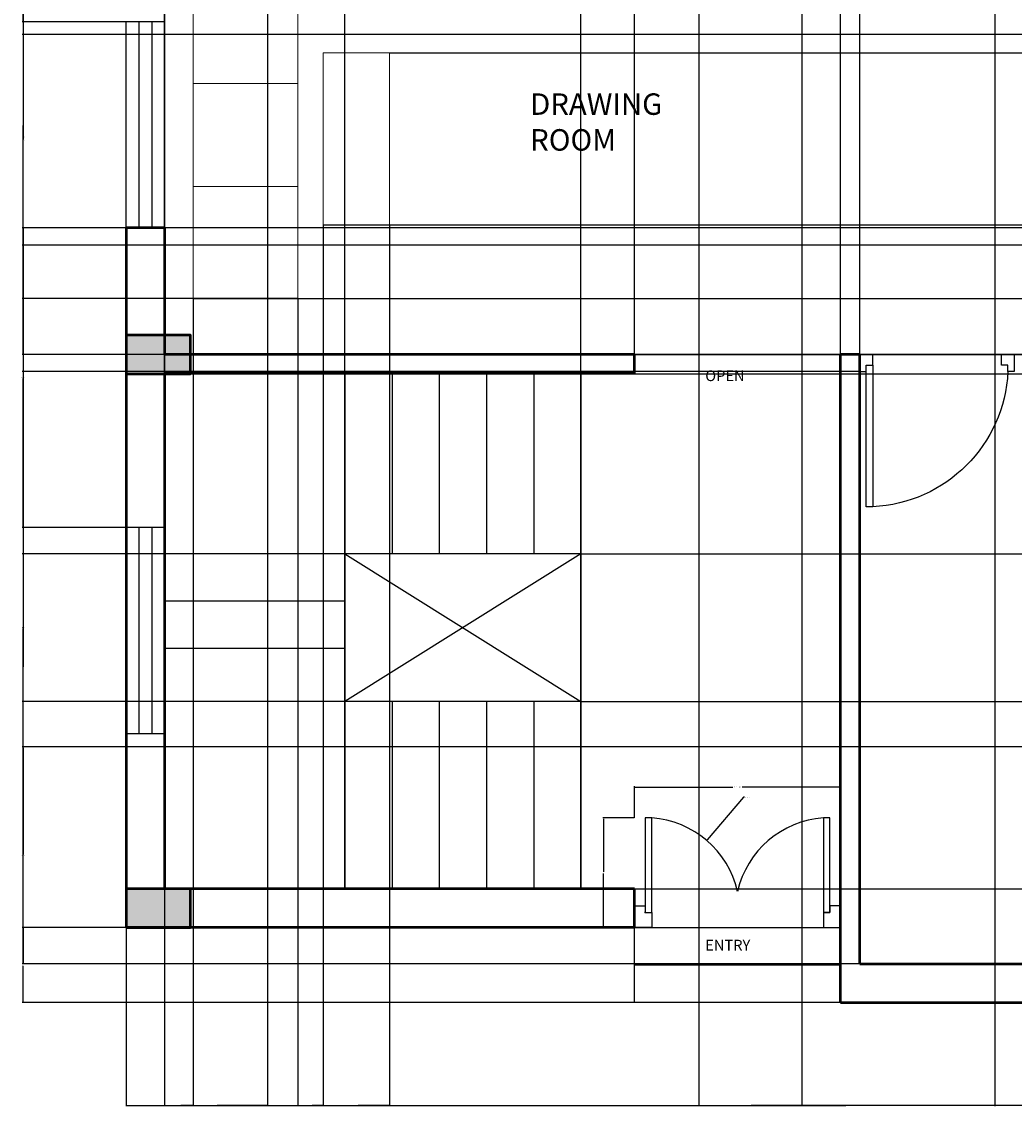
# Model space of a CAD drawing. Units: inches. Extents: x 2480 to 2840, y 795 to 1323.
# Tile 1 of 4: x 2480 to 2711, y 795 to 1047. Entities that reach past the tile are written whole.
import ezdxf

# ---------------------------------------------------------------- set-up
doc = ezdxf.new("R2010")
doc.units = ezdxf.units.IN
for name, color, linetype, lineweight in [('A-ANNO-DIMS', 2, 'Continuous', 18), ('A-ANNO-TEXT', 7, 'Continuous', 18), ('A-AREA-IDEN', 7, 'Continuous', 25), ('COLUMN', 240, 'Continuous', 50), ('door', 140, 'Continuous', 25), ('Furniture', 9, 'Continuous', 18), ('staircase', 50, 'Continuous', 25), ('wall', 7, 'Continuous', 50), ('window', 201, 'Continuous', 25)]:
    doc.layers.add(name, color=color, linetype=linetype, lineweight=lineweight)
doc.styles.get("Standard").update_dxf_attribs({"font": 'arial.ttf'})
doc.dimstyles.get("Standard").update_dxf_attribs({"dimtxt": 0.18, "dimasz": 0.18, "dimexe": 0.18, "dimexo": 0.0625, "dimgap": 0.09, "dimtad": 0, "dimtih": 1, "dimtoh": 1, "dimdec": 4, "dimzin": 0, "dimdsep": 46, "dimtxsty": 'Standard', "dimcen": 0.09, "dimadec": 0, "dimazin": 0, "dimtfac": 1, "dimtdec": 4, "dimtofl": 0, "dimtmove": 0, "dimatfit": 3, "dimfxl": 1, "dimtolj": 1, "dimtzin": 0, "dimarcsym": 0})

# ---------------------------------------------------------------- blocks, each defined once
blk = doc.blocks.new('d3')
at = {"layer": 'door'}
blk.add_line((3146.77, 1027.98), (3194.77, 1027.98), dxfattribs=at)
for points in [[(3149.27, 1031.48), (3150.77, 1031.48), (3150.77, 1053.48), (3149.27, 1053.48)], [(3190.77, 1031.48), (3192.27, 1031.48), (3192.27, 1053.48), (3190.77, 1053.48)]]:
    blk.add_lwpolyline(points, close=True, dxfattribs=at)
for points in [[(3150.77, 1027.98), (3146.77, 1027.98), (3146.77, 1032.98), (3149.27, 1032.98), (3149.27, 1031.48), (3150.77, 1031.48), (3150.77, 1027.98)], [(3190.77, 1027.98), (3194.77, 1027.98), (3194.77, 1032.98), (3192.27, 1032.98), (3192.27, 1031.48), (3190.77, 1031.48), (3190.77, 1027.98)]]:
    blk.add_lwpolyline(points, dxfattribs=at)
for centre, start, end in [((3149.27, 1031.48), 12.8362, 86.0995), ((3192.27, 1031.48), 93.9005, 167.1638)]:
    blk.add_arc(centre, 22.05, start, end, dxfattribs=at)
blk = doc.blocks.new('w1')
at = {"layer": 'window'}
for p, q in [((2922.2, 1100.57), (2922.2, 1052.57)), ((2925.2, 1100.57), (2925.2, 1052.57))]:
    blk.add_line(p, q, dxfattribs=at)
blk.add_lwpolyline([(2919.2, 1052.57), (2928.2, 1052.57), (2928.2, 1100.57), (2919.2, 1100.57)], close=True, dxfattribs=at)
blk = doc.blocks.new('d1')
at = {"layer": 'door'}
blk.add_line((3049.73, 1052.02), (3085.73, 1052.02), dxfattribs=at)
blk.add_lwpolyline([(3051.23, 1054.52), (3052.73, 1054.52), (3052.73, 1087.52), (3051.23, 1087.52)], close=True, dxfattribs=at)
for points in [[(3052.73, 1052.02), (3049.73, 1052.02), (3049.73, 1056.02), (3051.23, 1056.02), (3051.23, 1054.52), (3052.73, 1054.52), (3052.73, 1052.02)], [(3082.73, 1052.02), (3085.73, 1052.02), (3085.73, 1056.02), (3084.23, 1056.02), (3084.23, 1054.52), (3082.73, 1054.52), (3082.73, 1052.02)]]:
    blk.add_lwpolyline(points, dxfattribs=at)
blk.add_arc((3051.23, 1054.52), 33.03, 2.6026, 87.3974, dxfattribs=at)
blk = doc.blocks.new('C')
at = {"layer": 'COLUMN'}
h = blk.add_hatch(color=256, dxfattribs=at)
h.dxf.hatch_style = 1
h.paths.add_polyline_path([(3016.24, 1218.72), (3031.24, 1218.72), (3031.24, 1227.72), (3016.24, 1227.72)])
blk.add_lwpolyline([(3016.24, 1218.72), (3031.24, 1218.72), (3031.24, 1227.72), (3016.24, 1227.72)], close=True, dxfattribs=at)
blk = doc.blocks.new('*D22')
at = {"layer": 'A-ANNO-DIMS', "color": 0, "lineweight": -2, "transparency": 16777216}
for p, q in [((2622.45, 861.8), (2622.45, 869.12)), ((2622.63, 868.94), (2645.37, 868.94)), ((2670.27, 868.94), (2647.54, 868.94)), ((2670.45, 861.8), (2670.45, 869.12))]:
    blk.add_line(p, q, dxfattribs=at)
at = {"layer": 'A-ANNO-DIMS', "color": 0, "transparency": 16777216}
for points in [[(2622.63, 868.97), (2622.63, 868.91), (2622.45, 868.94)], [(2670.27, 868.97), (2670.27, 868.91), (2670.45, 868.94)]]:
    blk.add_solid(points, dxfattribs=at)
at = {"layer": 'Defpoints', "color": 0, "transparency": 16777216}
for p in [(2670.45, 868.94), (2622.45, 861.74), (2670.45, 861.74)]:
    blk.add_point(p, dxfattribs=at)
at = {"layer": 'A-ANNO-DIMS', "color": 0, "transparency": 16777216, "insert": (2646.45, 868.94), "char_height": 0.18, "attachment_point": 5}
blk.add_mtext('\\A1;ENTRY DOOR 48', dxfattribs=at)
blk = doc.blocks.new('*D23')
at = {"layer": 'A-ANNO-DIMS', "color": 0, "lineweight": -2, "transparency": 16777216}
for p, q in [((2622.39, 861.74), (2615.07, 861.74)), ((2615.25, 861.56), (2615.25, 849.17)), ((2615.25, 836.42), (2615.25, 848.81)), ((2622.39, 836.24), (2615.07, 836.24))]:
    blk.add_line(p, q, dxfattribs=at)
at = {"layer": 'A-ANNO-DIMS', "color": 0, "transparency": 16777216}
for points in [[(2615.22, 861.56), (2615.28, 861.56), (2615.25, 861.74)], [(2615.22, 836.42), (2615.28, 836.42), (2615.25, 836.24)]]:
    blk.add_solid(points, dxfattribs=at)
at = {"layer": 'Defpoints', "color": 0, "transparency": 16777216}
for p in [(2615.25, 861.74), (2622.45, 861.74), (2622.45, 836.24)]:
    blk.add_point(p, dxfattribs=at)
at = {"layer": 'A-ANNO-DIMS', "color": 0, "transparency": 16777216, "insert": (2615.25, 848.99), "char_height": 0.18, "attachment_point": 5}
blk.add_mtext('\\A1;26', dxfattribs=at)
blk = doc.blocks.new('*D28')
at = {"layer": 'A-ANNO-DIMS', "color": 0, "lineweight": -2, "transparency": 16777216}
for p, q in [((2503.95, 836.18), (2503.95, 794.56)), ((2815.95, 818.68), (2815.95, 794.56)), ((2504.13, 794.74), (2659.67, 794.74)), ((2815.77, 794.74), (2660.24, 794.74))]:
    blk.add_line(p, q, dxfattribs=at)
at = {"layer": 'A-ANNO-DIMS', "color": 0, "transparency": 16777216}
for points in [[(2504.13, 794.77), (2504.13, 794.71), (2503.95, 794.74)], [(2815.77, 794.77), (2815.77, 794.71), (2815.95, 794.74)]]:
    blk.add_solid(points, dxfattribs=at)
at = {"layer": 'Defpoints', "color": 0, "transparency": 16777216}
for p in [(2503.95, 836.24), (2815.95, 818.74), (2815.95, 794.74)]:
    blk.add_point(p, dxfattribs=at)
at = {"layer": 'A-ANNO-DIMS', "color": 0, "transparency": 16777216, "insert": (2659.95, 794.74), "char_height": 0.18, "attachment_point": 5}
blk.add_mtext('\\A1;312', dxfattribs=at)
blk = doc.blocks.new('*D35')
at = {"layer": 'A-ANNO-DIMS', "color": 0, "lineweight": -2, "transparency": 16777216}
for p, q in [((2503.89, 1105.24), (2479.77, 1105.24)), ((2479.95, 1105.06), (2479.95, 1076.42)), ((2479.95, 1047.42), (2479.95, 1076.06)), ((2503.89, 1047.24), (2479.77, 1047.24))]:
    blk.add_line(p, q, dxfattribs=at)
at = {"layer": 'A-ANNO-DIMS', "color": 0, "transparency": 16777216}
for points in [[(2479.92, 1105.06), (2479.98, 1105.06), (2479.95, 1105.24)], [(2479.92, 1047.42), (2479.98, 1047.42), (2479.95, 1047.24)]]:
    blk.add_solid(points, dxfattribs=at)
at = {"layer": 'Defpoints', "color": 0, "transparency": 16777216}
for p in [(2503.95, 1105.24), (2479.95, 1047.24), (2503.95, 1047.24)]:
    blk.add_point(p, dxfattribs=at)
at = {"layer": 'A-ANNO-DIMS', "color": 0, "transparency": 16777216, "insert": (2479.95, 1076.24), "char_height": 0.18, "attachment_point": 5}
blk.add_mtext('\\A1;58', dxfattribs=at)
blk = doc.blocks.new('*D36')
at = {"layer": 'A-ANNO-DIMS', "color": 0, "lineweight": -2, "transparency": 16777216}
for p, q in [((2503.89, 999.24), (2479.77, 999.24)), ((2479.95, 999.06), (2479.95, 964.51)), ((2479.95, 929.6), (2479.95, 964.15)), ((2503.89, 929.42), (2479.77, 929.42))]:
    blk.add_line(p, q, dxfattribs=at)
at = {"layer": 'A-ANNO-DIMS', "color": 0, "transparency": 16777216}
for points in [[(2479.92, 999.06), (2479.98, 999.06), (2479.95, 999.24)], [(2479.92, 929.6), (2479.98, 929.6), (2479.95, 929.42)]]:
    blk.add_solid(points, dxfattribs=at)
at = {"layer": 'Defpoints', "color": 0, "transparency": 16777216}
for p in [(2503.95, 999.24), (2479.95, 929.42), (2503.95, 929.42)]:
    blk.add_point(p, dxfattribs=at)
at = {"layer": 'A-ANNO-DIMS', "color": 0, "transparency": 16777216, "insert": (2479.95, 964.33), "char_height": 0.18, "attachment_point": 5}
blk.add_mtext('\\A1;69.82', dxfattribs=at)
blk = doc.blocks.new('*D37')
at = {"layer": 'A-ANNO-DIMS', "color": 0, "lineweight": -2, "transparency": 16777216}
for p, q in [((2806.89, 878.28), (2479.77, 878.28)), ((2479.95, 878.1), (2479.95, 853.19)), ((2479.95, 827.92), (2479.95, 852.83)), ((2806.89, 827.74), (2479.77, 827.74))]:
    blk.add_line(p, q, dxfattribs=at)
at = {"layer": 'A-ANNO-DIMS', "color": 0, "transparency": 16777216}
for points in [[(2479.92, 878.1), (2479.98, 878.1), (2479.95, 878.28)], [(2479.92, 827.92), (2479.98, 827.92), (2479.95, 827.74)]]:
    blk.add_solid(points, dxfattribs=at)
at = {"layer": 'Defpoints', "color": 0, "transparency": 16777216}
for p in [(2479.95, 878.28), (2806.95, 878.28), (2806.95, 827.74)]:
    blk.add_point(p, dxfattribs=at)
at = {"layer": 'A-ANNO-DIMS', "color": 0, "transparency": 16777216, "insert": (2479.95, 853.01), "char_height": 0.18, "attachment_point": 5}
blk.add_mtext('\\A1;50.53', dxfattribs=at)
blk = doc.blocks.new('*D38')
at = {"layer": 'A-ANNO-DIMS', "color": 0, "lineweight": -2, "transparency": 16777216}
for p, q in [((2806.89, 999.24), (2479.77, 999.24)), ((2479.95, 999.06), (2479.95, 984.67)), ((2479.95, 969.92), (2479.95, 984.31)), ((2806.89, 969.74), (2479.77, 969.74))]:
    blk.add_line(p, q, dxfattribs=at)
at = {"layer": 'A-ANNO-DIMS', "color": 0, "transparency": 16777216}
for points in [[(2479.92, 999.06), (2479.98, 999.06), (2479.95, 999.24)], [(2479.92, 969.92), (2479.98, 969.92), (2479.95, 969.74)]]:
    blk.add_solid(points, dxfattribs=at)
at = {"layer": 'Defpoints', "color": 0, "transparency": 16777216}
for p in [(2479.95, 999.24), (2806.95, 999.24), (2806.95, 969.74)]:
    blk.add_point(p, dxfattribs=at)
at = {"layer": 'A-ANNO-DIMS', "color": 0, "transparency": 16777216, "insert": (2479.95, 984.49), "char_height": 0.18, "attachment_point": 5}
blk.add_mtext('\\A1;29.5', dxfattribs=at)
blk = doc.blocks.new('*D42')
at = {"layer": 'A-ANNO-DIMS', "color": 0, "lineweight": -2, "transparency": 16777216}
for p, q in [((2512.95, 969.8), (2512.95, 1322.93)), ((2513.13, 1322.75), (2567.32, 1322.75)), ((2622.27, 1322.75), (2568.09, 1322.75)), ((2622.45, 969.8), (2622.45, 1322.93))]:
    blk.add_line(p, q, dxfattribs=at)
at = {"layer": 'A-ANNO-DIMS', "color": 0, "transparency": 16777216}
for points in [[(2513.13, 1322.78), (2513.13, 1322.72), (2512.95, 1322.75)], [(2622.27, 1322.78), (2622.27, 1322.72), (2622.45, 1322.75)]]:
    blk.add_solid(points, dxfattribs=at)
at = {"layer": 'Defpoints', "color": 0, "transparency": 16777216}
for p in [(2622.45, 1322.75), (2512.95, 969.74), (2622.45, 969.74)]:
    blk.add_point(p, dxfattribs=at)
at = {"layer": 'A-ANNO-DIMS', "color": 0, "transparency": 16777216, "insert": (2567.7, 1322.75), "char_height": 0.18, "attachment_point": 5}
blk.add_mtext('\\A1;109.5', dxfattribs=at)
blk = doc.blocks.new('*D43')
at = {"layer": 'A-ANNO-DIMS', "color": 0, "lineweight": -2, "transparency": 16777216}
for p, q in [((2622.39, 836.24), (2479.77, 836.24)), ((2479.95, 836.06), (2479.95, 827.67)), ((2479.95, 818.92), (2479.95, 827.31)), ((2622.39, 818.74), (2479.77, 818.74))]:
    blk.add_line(p, q, dxfattribs=at)
at = {"layer": 'A-ANNO-DIMS', "color": 0, "transparency": 16777216}
for points in [[(2479.92, 836.06), (2479.98, 836.06), (2479.95, 836.24)], [(2479.92, 818.92), (2479.98, 818.92), (2479.95, 818.74)]]:
    blk.add_solid(points, dxfattribs=at)
at = {"layer": 'Defpoints', "color": 0, "transparency": 16777216}
for p in [(2479.95, 836.24), (2622.45, 836.24), (2622.45, 818.74)]:
    blk.add_point(p, dxfattribs=at)
at = {"layer": 'A-ANNO-DIMS', "color": 0, "transparency": 16777216, "insert": (2479.95, 827.49), "char_height": 0.18, "attachment_point": 5}
blk.add_mtext('\\A1;17.5', dxfattribs=at)
blk = doc.blocks.new('*D44')
at = {"layer": 'A-ANNO-DIMS', "color": 0, "lineweight": -2, "transparency": 16777216}
for p, q in [((2706.39, 1076.74), (2479.77, 1076.74)), ((2479.95, 1076.56), (2479.95, 1023.42)), ((2479.95, 969.92), (2479.95, 1023.06)), ((2710.89, 969.74), (2479.77, 969.74))]:
    blk.add_line(p, q, dxfattribs=at)
at = {"layer": 'A-ANNO-DIMS', "color": 0, "transparency": 16777216}
for points in [[(2479.92, 1076.56), (2479.98, 1076.56), (2479.95, 1076.74)], [(2479.92, 969.92), (2479.98, 969.92), (2479.95, 969.74)]]:
    blk.add_solid(points, dxfattribs=at)
at = {"layer": 'Defpoints', "color": 0, "transparency": 16777216}
for p in [(2479.95, 1076.74), (2706.45, 1076.74), (2710.95, 969.74)]:
    blk.add_point(p, dxfattribs=at)
at = {"layer": 'A-ANNO-DIMS', "color": 0, "transparency": 16777216, "insert": (2479.95, 1023.24), "char_height": 0.18, "attachment_point": 5}
blk.add_mtext('\\A1;107', dxfattribs=at)
blk = doc.blocks.new('*D45')
at = {"layer": 'A-ANNO-DIMS', "color": 0, "lineweight": -2, "transparency": 16777216}
for p, q in [((2512.95, 923.3), (2512.95, 1322.93)), ((2513.13, 1322.75), (2533.73, 1322.75)), ((2554.77, 1322.75), (2534.18, 1322.75)), ((2554.95, 923.3), (2554.95, 1322.93))]:
    blk.add_line(p, q, dxfattribs=at)
at = {"layer": 'A-ANNO-DIMS', "color": 0, "transparency": 16777216}
for points in [[(2513.13, 1322.78), (2513.13, 1322.72), (2512.95, 1322.75)], [(2554.77, 1322.78), (2554.77, 1322.72), (2554.95, 1322.75)]]:
    blk.add_solid(points, dxfattribs=at)
at = {"layer": 'Defpoints', "color": 0, "transparency": 16777216}
for p in [(2554.95, 1322.75), (2512.95, 923.24), (2554.95, 923.24)]:
    blk.add_point(p, dxfattribs=at)
at = {"layer": 'A-ANNO-DIMS', "color": 0, "transparency": 16777216, "insert": (2533.95, 1322.75), "char_height": 0.18, "attachment_point": 5}
blk.add_mtext('\\A1;42', dxfattribs=at)
blk = doc.blocks.new('*D46')
at = {"layer": 'A-ANNO-DIMS', "color": 0, "lineweight": -2, "transparency": 16777216}
for p, q in [((2610.02, 888.87), (2840.14, 888.87)), ((2839.96, 888.69), (2839.96, 867.24)), ((2839.96, 845.42), (2839.96, 866.87)), ((2610.02, 845.24), (2840.14, 845.24))]:
    blk.add_line(p, q, dxfattribs=at)
at = {"layer": 'A-ANNO-DIMS', "color": 0, "transparency": 16777216}
for points in [[(2839.93, 888.69), (2839.99, 888.69), (2839.96, 888.87)], [(2839.93, 845.42), (2839.99, 845.42), (2839.96, 845.24)]]:
    blk.add_solid(points, dxfattribs=at)
at = {"layer": 'Defpoints', "color": 0, "transparency": 16777216}
for p in [(2609.95, 888.87), (2839.96, 888.87), (2609.95, 845.24)]:
    blk.add_point(p, dxfattribs=at)
at = {"layer": 'A-ANNO-DIMS', "color": 0, "transparency": 16777216, "insert": (2839.96, 867.06), "char_height": 0.18, "attachment_point": 5}
blk.add_mtext('\\A1;43.63', dxfattribs=at)
blk = doc.blocks.new('*D47')
at = {"layer": 'A-ANNO-DIMS', "color": 0, "lineweight": -2, "transparency": 16777216}
for p, q in [((2554.95, 845.3), (2554.95, 1322.93)), ((2555.13, 1322.75), (2582.23, 1322.75)), ((2609.77, 1322.75), (2582.67, 1322.75)), ((2609.95, 845.3), (2609.95, 1322.93))]:
    blk.add_line(p, q, dxfattribs=at)
at = {"layer": 'A-ANNO-DIMS', "color": 0, "transparency": 16777216}
for points in [[(2555.13, 1322.78), (2555.13, 1322.72), (2554.95, 1322.75)], [(2609.77, 1322.78), (2609.77, 1322.72), (2609.95, 1322.75)]]:
    blk.add_solid(points, dxfattribs=at)
at = {"layer": 'Defpoints', "color": 0, "transparency": 16777216}
for p in [(2609.95, 1322.75), (2554.95, 845.24), (2609.95, 845.24)]:
    blk.add_point(p, dxfattribs=at)
at = {"layer": 'A-ANNO-DIMS', "color": 0, "transparency": 16777216, "insert": (2582.45, 1322.75), "char_height": 0.18, "attachment_point": 5}
blk.add_mtext('\\A1;55', dxfattribs=at)
blk = doc.blocks.new('*D48')
at = {"layer": 'A-ANNO-DIMS', "color": 0, "lineweight": -2, "transparency": 16777216}
for p, q in [((2554.89, 923.24), (2479.77, 923.24)), ((2479.95, 923.06), (2479.95, 906.24)), ((2479.95, 889.05), (2479.95, 905.87)), ((2554.89, 888.87), (2479.77, 888.87))]:
    blk.add_line(p, q, dxfattribs=at)
at = {"layer": 'A-ANNO-DIMS', "color": 0, "transparency": 16777216}
for points in [[(2479.92, 923.06), (2479.98, 923.06), (2479.95, 923.24)], [(2479.92, 889.05), (2479.98, 889.05), (2479.95, 888.87)]]:
    blk.add_solid(points, dxfattribs=at)
at = {"layer": 'Defpoints', "color": 0, "transparency": 16777216}
for p in [(2479.95, 923.24), (2554.95, 923.24), (2554.95, 888.87)]:
    blk.add_point(p, dxfattribs=at)
at = {"layer": 'A-ANNO-DIMS', "color": 0, "transparency": 16777216, "insert": (2479.95, 906.06), "char_height": 0.18, "attachment_point": 5}
blk.add_mtext('\\A1;34.37', dxfattribs=at)
blk = doc.blocks.new('*D49')
at = {"layer": 'A-ANNO-DIMS', "color": 0, "lineweight": -2, "transparency": 16777216}
for p, q in [((2610.02, 965.24), (2840.14, 965.24)), ((2839.96, 965.06), (2839.96, 944.42)), ((2839.96, 923.42), (2839.96, 944.06)), ((2610.02, 923.24), (2840.14, 923.24))]:
    blk.add_line(p, q, dxfattribs=at)
at = {"layer": 'A-ANNO-DIMS', "color": 0, "transparency": 16777216}
for points in [[(2839.93, 965.06), (2839.99, 965.06), (2839.96, 965.24)], [(2839.93, 923.42), (2839.99, 923.42), (2839.96, 923.24)]]:
    blk.add_solid(points, dxfattribs=at)
at = {"layer": 'Defpoints', "color": 0, "transparency": 16777216}
for p in [(2609.95, 965.24), (2839.96, 965.24), (2609.95, 923.24)]:
    blk.add_point(p, dxfattribs=at)
at = {"layer": 'A-ANNO-DIMS', "color": 0, "transparency": 16777216, "insert": (2839.96, 944.24), "char_height": 0.18, "attachment_point": 5}
blk.add_mtext('\\A1;42', dxfattribs=at)
blk = doc.blocks.new('*D50')
at = {"layer": 'A-ANNO-DIMS', "color": 0, "lineweight": -2, "transparency": 16777216}
for p, q in [((2637.45, 1076.68), (2637.45, 794.56)), ((2706.45, 1076.68), (2706.45, 794.56)), ((2637.63, 794.74), (2671.73, 794.74)), ((2706.27, 794.74), (2672.17, 794.74))]:
    blk.add_line(p, q, dxfattribs=at)
at = {"layer": 'A-ANNO-DIMS', "color": 0, "transparency": 16777216}
for points in [[(2637.63, 794.77), (2637.63, 794.71), (2637.45, 794.74)], [(2706.27, 794.77), (2706.27, 794.71), (2706.45, 794.74)]]:
    blk.add_solid(points, dxfattribs=at)
at = {"layer": 'Defpoints', "color": 0, "transparency": 16777216}
for p in [(2637.45, 1076.74), (2706.45, 1076.74), (2706.45, 794.74)]:
    blk.add_point(p, dxfattribs=at)
at = {"layer": 'A-ANNO-DIMS', "color": 0, "transparency": 16777216, "insert": (2671.95, 794.74), "char_height": 0.18, "attachment_point": 5}
blk.add_mtext('\\A1;69', dxfattribs=at)
blk = doc.blocks.new('*D52')
at = {"layer": 'A-ANNO-DIMS', "color": 0, "lineweight": -2, "transparency": 16777216}
for p, q in [((2670.45, 818.8), (2670.45, 1322.93)), ((2670.63, 1322.75), (2672.45, 1322.75)), ((2674.77, 1322.75), (2672.96, 1322.75)), ((2674.95, 827.8), (2674.95, 1322.93))]:
    blk.add_line(p, q, dxfattribs=at)
at = {"layer": 'A-ANNO-DIMS', "color": 0, "transparency": 16777216}
for points in [[(2670.63, 1322.78), (2670.63, 1322.72), (2670.45, 1322.75)], [(2674.77, 1322.78), (2674.77, 1322.72), (2674.95, 1322.75)]]:
    blk.add_solid(points, dxfattribs=at)
at = {"layer": 'Defpoints', "color": 0, "transparency": 16777216}
for p in [(2674.95, 1322.75), (2674.95, 827.74), (2670.45, 818.74)]:
    blk.add_point(p, dxfattribs=at)
at = {"layer": 'A-ANNO-DIMS', "color": 0, "transparency": 16777216, "insert": (2672.7, 1322.75), "char_height": 0.18, "attachment_point": 5}
blk.add_mtext('\\A1;4.5', dxfattribs=at)
blk = doc.blocks.new('*D53')
at = {"layer": 'A-ANNO-DIMS', "color": 0, "lineweight": -2, "transparency": 16777216}
for p, q in [((2565.4, 1040.02), (2840.14, 1040.02)), ((2839.96, 1039.84), (2839.96, 1020.15)), ((2839.96, 1000.1), (2839.96, 1019.79)), ((2565.4, 999.92), (2840.14, 999.92))]:
    blk.add_line(p, q, dxfattribs=at)
at = {"layer": 'A-ANNO-DIMS', "color": 0, "transparency": 16777216}
for points in [[(2839.93, 1039.84), (2839.99, 1039.84), (2839.96, 1040.02)], [(2839.93, 1000.1), (2839.99, 1000.1), (2839.96, 999.92)]]:
    blk.add_solid(points, dxfattribs=at)
at = {"layer": 'Defpoints', "color": 0, "transparency": 16777216}
for p in [(2565.34, 1040.02), (2839.96, 1040.02), (2565.34, 999.92)]:
    blk.add_point(p, dxfattribs=at)
at = {"layer": 'A-ANNO-DIMS', "color": 0, "transparency": 16777216, "insert": (2839.96, 1019.97), "char_height": 0.18, "attachment_point": 5}
blk.add_mtext('\\A1;40.1', dxfattribs=at)
blk = doc.blocks.new('*D55')
at = {"layer": 'A-ANNO-DIMS', "color": 0, "lineweight": -2, "transparency": 16777216}
for p, q in [((2543.94, 1058.07), (2479.77, 1058.07)), ((2479.95, 1057.89), (2479.95, 1020.58)), ((2479.95, 982.91), (2479.95, 1020.21)), ((2543.94, 982.73), (2479.77, 982.73))]:
    blk.add_line(p, q, dxfattribs=at)
at = {"layer": 'A-ANNO-DIMS', "color": 0, "transparency": 16777216}
for points in [[(2479.92, 1057.89), (2479.98, 1057.89), (2479.95, 1058.07)], [(2479.92, 982.91), (2479.98, 982.91), (2479.95, 982.73)]]:
    blk.add_solid(points, dxfattribs=at)
at = {"layer": 'Defpoints', "color": 0, "transparency": 16777216}
for p in [(2479.95, 1058.07), (2544, 1058.07), (2544, 982.73)]:
    blk.add_point(p, dxfattribs=at)
at = {"layer": 'A-ANNO-DIMS', "color": 0, "transparency": 16777216, "insert": (2479.95, 1020.4), "char_height": 0.18, "attachment_point": 5}
blk.add_mtext('\\A1;75.34', dxfattribs=at)
blk = doc.blocks.new('*D56')
at = {"layer": 'A-ANNO-DIMS', "color": 0, "lineweight": -2, "transparency": 16777216}
for p, q in [((2549.93, 999.86), (2549.93, 794.56)), ((2565.34, 999.86), (2565.34, 794.56)), ((2550.11, 794.74), (2557.18, 794.74)), ((2565.16, 794.74), (2558.09, 794.74))]:
    blk.add_line(p, q, dxfattribs=at)
at = {"layer": 'A-ANNO-DIMS', "color": 0, "transparency": 16777216}
for points in [[(2550.11, 794.77), (2550.11, 794.71), (2549.93, 794.74)], [(2565.16, 794.77), (2565.16, 794.71), (2565.34, 794.74)]]:
    blk.add_solid(points, dxfattribs=at)
at = {"layer": 'Defpoints', "color": 0, "transparency": 16777216}
for p in [(2549.93, 999.92), (2565.34, 999.92), (2565.34, 794.74)]:
    blk.add_point(p, dxfattribs=at)
at = {"layer": 'A-ANNO-DIMS', "color": 0, "transparency": 16777216, "insert": (2557.64, 794.74), "char_height": 0.18, "attachment_point": 5}
blk.add_mtext('\\A1;15.408', dxfattribs=at)
blk = doc.blocks.new('*D58')
at = {"layer": 'A-ANNO-DIMS', "color": 0, "lineweight": -2, "transparency": 16777216}
for p, q in [((2799.14, 1044.23), (2479.77, 1044.23)), ((2479.95, 1044.05), (2479.95, 1019.89)), ((2479.95, 995.36), (2479.95, 1019.52)), ((2799.14, 995.18), (2479.77, 995.18))]:
    blk.add_line(p, q, dxfattribs=at)
at = {"layer": 'A-ANNO-DIMS', "color": 0, "transparency": 16777216}
for points in [[(2479.92, 1044.05), (2479.98, 1044.05), (2479.95, 1044.23)], [(2479.92, 995.36), (2479.98, 995.36), (2479.95, 995.18)]]:
    blk.add_solid(points, dxfattribs=at)
at = {"layer": 'Defpoints', "color": 0, "transparency": 16777216}
for p in [(2479.95, 1044.23), (2799.2, 1044.23), (2799.2, 995.18)]:
    blk.add_point(p, dxfattribs=at)
at = {"layer": 'A-ANNO-DIMS', "color": 0, "transparency": 16777216, "insert": (2479.95, 1019.7), "char_height": 0.18, "attachment_point": 5}
blk.add_mtext('\\A1;49.06', dxfattribs=at)
blk = doc.blocks.new('*D59')
at = {"layer": 'A-ANNO-DIMS', "color": 0, "lineweight": -2, "transparency": 16777216}
for p, q in [((2519.64, 982.66), (2519.64, 794.56)), ((2512.95, 969.68), (2512.95, 794.56)), ((2513.13, 794.74), (2515.9, 794.74)), ((2519.46, 794.74), (2516.69, 794.74))]:
    blk.add_line(p, q, dxfattribs=at)
at = {"layer": 'A-ANNO-DIMS', "color": 0, "transparency": 16777216}
for points in [[(2513.13, 794.77), (2513.13, 794.71), (2512.95, 794.74)], [(2519.46, 794.77), (2519.46, 794.71), (2519.64, 794.74)]]:
    blk.add_solid(points, dxfattribs=at)
at = {"layer": 'Defpoints', "color": 0, "transparency": 16777216}
for p in [(2519.64, 982.73), (2512.95, 969.74), (2519.64, 794.74)]:
    blk.add_point(p, dxfattribs=at)
at = {"layer": 'A-ANNO-DIMS', "color": 0, "transparency": 16777216, "insert": (2516.3, 794.74), "char_height": 0.18, "attachment_point": 5}
blk.add_mtext('\\A1;6.686', dxfattribs=at)
blk = doc.blocks.new('*D60')
at = {"layer": 'A-ANNO-DIMS', "color": 0, "lineweight": -2, "transparency": 16777216}
for p, q in [((2519.7, 982.73), (2840.14, 982.73)), ((2839.96, 982.55), (2839.96, 976.42)), ((2839.96, 969.92), (2839.96, 976.05)), ((2513.02, 969.74), (2840.14, 969.74))]:
    blk.add_line(p, q, dxfattribs=at)
at = {"layer": 'A-ANNO-DIMS', "color": 0, "transparency": 16777216}
for points in [[(2839.93, 982.55), (2839.99, 982.55), (2839.96, 982.73)], [(2839.93, 969.92), (2839.99, 969.92), (2839.96, 969.74)]]:
    blk.add_solid(points, dxfattribs=at)
at = {"layer": 'Defpoints', "color": 0, "transparency": 16777216}
for p in [(2519.64, 982.73), (2839.96, 982.73), (2512.95, 969.74)]:
    blk.add_point(p, dxfattribs=at)
at = {"layer": 'A-ANNO-DIMS', "color": 0, "transparency": 16777216, "insert": (2839.96, 976.23), "char_height": 0.18, "attachment_point": 5}
blk.add_mtext('\\A1;12.984', dxfattribs=at)
blk = doc.blocks.new('*D63')
at = {"layer": 'A-ANNO-DIMS', "color": 0, "lineweight": -2, "transparency": 16777216}
for p, q in [((2549.93, 999.86), (2549.93, 794.56)), ((2544, 982.66), (2544, 794.56)), ((2544.18, 794.74), (2546.57, 794.74)), ((2549.75, 794.74), (2547.36, 794.74))]:
    blk.add_line(p, q, dxfattribs=at)
at = {"layer": 'A-ANNO-DIMS', "color": 0, "transparency": 16777216}
for points in [[(2544.18, 794.77), (2544.18, 794.71), (2544, 794.74)], [(2549.75, 794.77), (2549.75, 794.71), (2549.93, 794.74)]]:
    blk.add_solid(points, dxfattribs=at)
at = {"layer": 'Defpoints', "color": 0, "transparency": 16777216}
for p in [(2549.93, 999.92), (2544, 982.73), (2549.93, 794.74)]:
    blk.add_point(p, dxfattribs=at)
at = {"layer": 'A-ANNO-DIMS', "color": 0, "transparency": 16777216, "insert": (2546.97, 794.74), "char_height": 0.18, "attachment_point": 5}
blk.add_mtext('\\A1;5.929', dxfattribs=at)
blk = doc.blocks.new('*D64')
at = {"layer": 'A-ANNO-DIMS', "color": 0, "lineweight": -2, "transparency": 16777216}
for p, q in [((2550, 999.92), (2840.14, 999.92)), ((2839.96, 999.74), (2839.96, 991.5)), ((2839.96, 982.91), (2839.96, 991.14)), ((2544.07, 982.73), (2840.14, 982.73))]:
    blk.add_line(p, q, dxfattribs=at)
at = {"layer": 'A-ANNO-DIMS', "color": 0, "transparency": 16777216}
for points in [[(2839.93, 999.74), (2839.99, 999.74), (2839.96, 999.92)], [(2839.93, 982.91), (2839.99, 982.91), (2839.96, 982.73)]]:
    blk.add_solid(points, dxfattribs=at)
at = {"layer": 'Defpoints', "color": 0, "transparency": 16777216}
for p in [(2549.93, 999.92), (2839.96, 999.92), (2544, 982.73)]:
    blk.add_point(p, dxfattribs=at)
at = {"layer": 'A-ANNO-DIMS', "color": 0, "transparency": 16777216, "insert": (2839.96, 991.32), "char_height": 0.18, "attachment_point": 5}
blk.add_mtext('\\A1;17.193', dxfattribs=at)
blk = doc.blocks.new('*D65')
at = {"layer": 'A-ANNO-DIMS', "color": 0, "lineweight": -2, "transparency": 16777216}
for p, q in [((2512.95, 1289.68), (2512.95, 794.56)), ((2536.95, 1289.68), (2536.95, 794.56)), ((2513.13, 794.74), (2524.73, 794.74)), ((2536.77, 794.74), (2525.17, 794.74))]:
    blk.add_line(p, q, dxfattribs=at)
at = {"layer": 'A-ANNO-DIMS', "color": 0, "transparency": 16777216}
for points in [[(2513.13, 794.77), (2513.13, 794.71), (2512.95, 794.74)], [(2536.77, 794.77), (2536.77, 794.71), (2536.95, 794.74)]]:
    blk.add_solid(points, dxfattribs=at)
at = {"layer": 'Defpoints', "color": 0, "transparency": 16777216}
for p in [(2512.95, 1289.74), (2536.95, 1289.74), (2536.95, 794.74)]:
    blk.add_point(p, dxfattribs=at)
at = {"layer": 'A-ANNO-DIMS', "color": 0, "transparency": 16777216, "insert": (2524.95, 794.74), "char_height": 0.18, "attachment_point": 5}
blk.add_mtext('\\A1;24', dxfattribs=at)
blk = doc.blocks.new('*D66')
at = {"layer": 'A-ANNO-DIMS', "color": 0, "lineweight": -2, "transparency": 16777216}
for p, q in [((2637.45, 1289.68), (2637.45, 794.56)), ((2661.45, 1289.68), (2661.45, 794.56)), ((2637.63, 794.74), (2649.23, 794.74)), ((2661.27, 794.74), (2649.67, 794.74))]:
    blk.add_line(p, q, dxfattribs=at)
at = {"layer": 'A-ANNO-DIMS', "color": 0, "transparency": 16777216}
for points in [[(2637.63, 794.77), (2637.63, 794.71), (2637.45, 794.74)], [(2661.27, 794.77), (2661.27, 794.71), (2661.45, 794.74)]]:
    blk.add_solid(points, dxfattribs=at)
at = {"layer": 'Defpoints', "color": 0, "transparency": 16777216}
for p in [(2637.45, 1289.74), (2661.45, 1289.74), (2661.45, 794.74)]:
    blk.add_point(p, dxfattribs=at)
at = {"layer": 'A-ANNO-DIMS', "color": 0, "transparency": 16777216, "insert": (2649.45, 794.74), "char_height": 0.18, "attachment_point": 5}
blk.add_mtext('\\A1;24', dxfattribs=at)
blk = doc.blocks.new('*D67')
at = {"layer": 'A-ANNO-DIMS', "color": 0, "lineweight": -2, "transparency": 16777216}
for p, q in [((2674.95, 827.8), (2674.95, 1322.93)), ((2675.13, 1322.75), (2694.94, 1322.75)), ((2715.53, 1322.75), (2695.73, 1322.75)), ((2715.71, 827.8), (2715.71, 1322.93))]:
    blk.add_line(p, q, dxfattribs=at)
at = {"layer": 'A-ANNO-DIMS', "color": 0, "transparency": 16777216}
for points in [[(2675.13, 1322.78), (2675.13, 1322.72), (2674.95, 1322.75)], [(2715.53, 1322.78), (2715.53, 1322.72), (2715.71, 1322.75)]]:
    blk.add_solid(points, dxfattribs=at)
at = {"layer": 'Defpoints', "color": 0, "transparency": 16777216}
for p in [(2715.71, 1322.75), (2674.95, 827.74), (2715.71, 827.74)]:
    blk.add_point(p, dxfattribs=at)
at = {"layer": 'A-ANNO-DIMS', "color": 0, "transparency": 16777216, "insert": (2695.33, 1322.75), "char_height": 0.18, "attachment_point": 5}
blk.add_mtext('\\A1;40.76', dxfattribs=at)
blk = doc.blocks.new('*D68')
at = {"layer": 'A-ANNO-DIMS', "color": 0, "lineweight": -2, "transparency": 16777216}
for p, q in [((2674.89, 965.74), (2479.77, 965.74)), ((2479.95, 965.56), (2479.95, 896.92)), ((2479.95, 827.92), (2479.95, 896.56)), ((2674.89, 827.74), (2479.77, 827.74))]:
    blk.add_line(p, q, dxfattribs=at)
at = {"layer": 'A-ANNO-DIMS', "color": 0, "transparency": 16777216}
for points in [[(2479.92, 965.56), (2479.98, 965.56), (2479.95, 965.74)], [(2479.92, 827.92), (2479.98, 827.92), (2479.95, 827.74)]]:
    blk.add_solid(points, dxfattribs=at)
at = {"layer": 'Defpoints', "color": 0, "transparency": 16777216}
for p in [(2479.95, 965.74), (2674.95, 965.74), (2674.95, 827.74)]:
    blk.add_point(p, dxfattribs=at)
at = {"layer": 'A-ANNO-DIMS', "color": 0, "transparency": 16777216, "insert": (2479.95, 896.74), "char_height": 0.18, "attachment_point": 5}
blk.add_mtext('\\A1;138', dxfattribs=at)
blk = doc.blocks.new('*D71')
at = {"layer": 'A-ANNO-DIMS', "color": 0, "lineweight": -2, "transparency": 16777216}
for p, q in [((2647.88, 866.56), (2639.4, 856.64)), ((2648.06, 866.56), (2647.88, 866.56)), ((2624.86, 839.74), (2625.04, 839.74)), ((2624.95, 839.65), (2624.95, 839.83))]:
    blk.add_line(p, q, dxfattribs=at)
at = {"layer": 'A-ANNO-DIMS', "color": 0, "transparency": 16777216}
blk.add_solid([(2639.38, 856.66), (2639.42, 856.62), (2639.28, 856.5)], dxfattribs=at)
at = {"layer": 'Defpoints', "color": 0, "transparency": 16777216}
for p in [(2639.28, 856.5), (2624.95, 839.74)]:
    blk.add_point(p, dxfattribs=at)
at = {"layer": 'A-ANNO-DIMS', "color": 0, "transparency": 16777216, "insert": (2648.74, 866.56), "char_height": 0.18, "attachment_point": 5}
blk.add_mtext('\\A1;2X R22.05', dxfattribs=at)

msp = doc.modelspace()

# ---------------------------------------------------------------- linework, layer by layer
at = {"layer": 'Furniture'}
for p, q in [((2519.6396, 1032.8713), (2544.0036, 1032.8713)), ((2519.6396, 1008.883), (2544.0036, 1008.883))]:
    msp.add_line(p, q, dxfattribs=at)
for points in [[(2519.6396, 1058.0677), (2544.0036, 1058.0677), (2544.0036, 982.726), (2519.6396, 982.726)], [(2549.9325, 1040.0192), (2565.3407, 1040.0192), (2565.3407, 999.9194), (2549.9325, 999.9194)]]:
    msp.add_lwpolyline(points, close=True, dxfattribs=at)
at = {"layer": 'staircase'}
for p, q in [((2554.9535, 965.2416), (2554.9535, 845.2416)), ((2565.9535, 965.2416), (2565.9535, 923.2416)), ((2576.9535, 965.2416), (2576.9535, 923.2416)), ((2587.9535, 965.2416), (2587.9535, 923.2416)), ((2598.9535, 965.2416), (2598.9535, 923.2416)), ((2609.9535, 965.2416), (2609.9535, 845.2416)), ((2609.9535, 923.2416), (2512.9535, 923.2416)), ((2554.9535, 923.2416), (2609.9535, 888.8711)), ((2609.9535, 923.2416), (2554.9535, 888.8711)), ((2554.9535, 912.2416), (2512.9535, 912.2416)), ((2554.9535, 901.2416), (2512.9535, 901.2416)), ((2609.9535, 888.8711), (2512.9535, 888.8711)), ((2565.9535, 888.8711), (2565.9535, 845.2416)), ((2576.9535, 888.8711), (2576.9535, 845.2416)), ((2587.9535, 888.8711), (2587.9535, 845.2416)), ((2598.9535, 888.8711), (2598.9535, 845.2416)), ((2622.4535, 827.4916), (2670.4535, 827.4916))]:
    msp.add_line(p, q, dxfattribs=at)
msp.add_lwpolyline([(2622.4535, 836.2416), (2670.4535, 836.2416), (2670.4535, 818.7416), (2622.4535, 818.7416)], close=True, dxfattribs=at)
at = {"layer": 'wall'}
for p, q in [((2512.9535, 999.2416), (2503.9535, 999.2416)), ((2503.9535, 999.2416), (2503.9535, 836.2416)), ((2512.9535, 999.2416), (2512.9535, 969.7416)), ((2622.4535, 969.7416), (2512.9535, 969.7416)), ((2622.4535, 965.2416), (2622.4535, 969.7416)), ((2670.4535, 818.7416), (2670.4535, 969.7416)), ((2674.9535, 969.7416), (2670.4535, 969.7416)), ((2674.9535, 827.7416), (2674.9535, 969.7416)), ((2512.9535, 965.2416), (2512.9535, 845.2416)), ((2622.4535, 965.2416), (2512.9535, 965.2416)), ((2622.4535, 845.2416), (2512.9535, 845.2416)), ((2622.4535, 836.2416), (2622.4535, 845.2416)), ((2622.4535, 836.2416), (2503.9535, 836.2416)), ((2674.9535, 827.7416), (2806.9535, 827.7416)), ((2670.4535, 818.7416), (2815.9535, 818.7416))]:
    msp.add_line(p, q, dxfattribs=at)

# ---------------------------------------------------------------- block references
at = {"layer": 'COLUMN'}
for p in [(-512.279, -253.4817), (-512.2865, -382.4817)]:
    msp.add_blockref('C', p, dxfattribs=at)
at = {"layer": 'door', "xscale": -1, "rotation": 180}
msp.add_blockref('d1', (-374.7789, 2021.7615), dxfattribs=at)
at = {"layer": 'door'}
msp.add_blockref('d3', (-524.3116, -191.7407), dxfattribs=at)
at = {"layer": 'window'}
for p in [(-415.2506, -53.327), (-415.2506, -171.1509)]:
    msp.add_blockref('w1', p, dxfattribs=at)

# ---------------------------------------------------------------- texts
at = {"layer": 'A-ANNO-TEXT', "char_height": 2.5, "attachment_point": 1}
for s, insert in [('OPEN', (2638.931, 966.003)), ('ENTRY', (2638.931, 833.3543))]:
    msp.add_mtext_dynamic_manual_height_columns(s, width=18.455809, gutter_width=12.5, heights=[0], dxfattribs=dict(at, insert=insert))
at = {"layer": 'A-AREA-IDEN', "insert": (2598.1366, 1030.5385), "char_height": 5, "attachment_point": 1}
msp.add_mtext_dynamic_manual_height_columns('DRAWING ROOM', width=47.7919, gutter_width=12.5, heights=[0], dxfattribs=at)

# ---------------------------------------------------------------- dimensions: what is measured, and where the dimension line sits
at = {"layer": 'A-ANNO-DIMS'}
for base, p1, p2, override, picture, middle in [((2622.4535, 1322.7466), (2512.9535, 969.7416), (2622.4535, 969.7416), {"dimdec": 1, "dimlfac": 1, "dimrnd": 0, "dimzin": 0, "dimdsep": 46, "dimlunit": 2}, '*D42', (2567.7035, 1322.7466)), ((2554.9535, 1322.7466), (2512.9535, 923.2416), (2554.9535, 923.2416), {"dimdec": 0, "dimlfac": 1, "dimrnd": 0, "dimzin": 0, "dimdsep": 46, "dimlunit": 2}, '*D45', (2533.9535, 1322.7466)), ((2609.9535, 1322.7466), (2554.9535, 845.2416), (2609.9535, 845.2416), {"dimdec": 0, "dimlfac": 1, "dimrnd": 0, "dimzin": 0, "dimdsep": 46, "dimlunit": 2}, '*D47', (2582.4535, 1322.7466)), ((2674.9535, 1322.7466), (2670.4535, 818.7416), (2674.9535, 827.7416), {"dimdec": 1, "dimlfac": 1, "dimrnd": 0, "dimzin": 0, "dimdsep": 46, "dimlunit": 2}, '*D52', (2672.7035, 1322.7466)), ((2715.7148, 1322.7466), (2674.9535, 827.7416), (2715.7148, 827.7416), {"dimdec": 2, "dimlfac": 1, "dimrnd": 0, "dimzin": 0, "dimdsep": 46, "dimlunit": 2}, '*D67', (2695.3342, 1322.7466)), ((2536.9535, 794.7366), (2512.9535, 1289.7416), (2536.9535, 1289.7416), {"dimdec": 0, "dimlfac": 1, "dimrnd": 0, "dimzin": 0, "dimdsep": 46, "dimlunit": 2}, '*D65', (2524.9535, 794.7366)), ((2661.4535, 794.7366), (2637.4535, 1289.7416), (2661.4535, 1289.7416), {"dimdec": 0, "dimlfac": 1, "dimrnd": 0, "dimzin": 0, "dimdsep": 46, "dimlunit": 2}, '*D66', (2649.4535, 794.7366)), ((2706.4535, 794.7366), (2637.4535, 1076.7416), (2706.4535, 1076.7416), {"dimdec": 0, "dimlfac": 1, "dimrnd": 0, "dimzin": 0, "dimdsep": 46, "dimlunit": 2}, '*D50', (2671.9535, 794.7366)), ((2549.9325, 794.7366), (2544.0036, 982.726), (2549.9325, 999.9194), {"dimdec": 3, "dimlfac": 1, "dimrnd": 0, "dimzin": 0, "dimdsep": 46, "dimlunit": 2}, '*D63', (2546.9681, 794.7366)), ((2565.3407, 794.7366), (2549.9325, 999.9194), (2565.3407, 999.9194), {"dimdec": 3, "dimlfac": 1, "dimrnd": 0, "dimzin": 0, "dimdsep": 46, "dimlunit": 2}, '*D56', (2557.6366, 794.7366)), ((2519.6396, 794.7366), (2512.9535, 969.7416), (2519.6396, 982.726), {"dimdec": 3, "dimlfac": 1, "dimrnd": 0, "dimzin": 0, "dimdsep": 46, "dimlunit": 2}, '*D59', (2516.2966, 794.7366)), ((2815.9535, 794.7366), (2503.9535, 836.2416), (2815.9535, 818.7416), {"dimdec": 0, "dimlfac": 1, "dimrnd": 0, "dimzin": 0, "dimdsep": 46, "dimlunit": 2}, '*D28', (2659.9535, 794.7366))]:
    dim = msp.add_linear_dim(base=base, p1=p1, p2=p2, dimstyle='Standard', override=override, dxfattribs=at)
    dim.commit()
    dim.dimension.update_dxf_attribs({"geometry": picture, "text_midpoint": middle})
for base, p1, p2, override, picture, middle in [((2479.9485, 1047.2416), (2503.9535, 1105.2416), (2503.9535, 1047.2416), {"dimdec": 0, "dimlfac": 1, "dimrnd": 0, "dimzin": 0, "dimdsep": 46, "dimlunit": 2}, '*D35', (2479.9485, 1076.2416)), ((2479.9485, 1076.7416), (2710.9535, 969.7416), (2706.4535, 1076.7416), {"dimdec": 0, "dimlfac": 1, "dimrnd": 0, "dimzin": 0, "dimdsep": 46, "dimlunit": 2}, '*D44', (2479.9485, 1023.2416)), ((2479.9485, 1058.0677), (2544.0036, 982.726), (2544.0036, 1058.0677), {"dimdec": 2, "dimlfac": 1, "dimrnd": 0, "dimzin": 0, "dimdsep": 46, "dimlunit": 2}, '*D55', (2479.9485, 1020.3968)), ((2479.9485, 1044.2327), (2799.2019, 995.1772), (2799.2019, 1044.2327), {"dimdec": 2, "dimlfac": 1, "dimrnd": 0, "dimzin": 0, "dimdsep": 46, "dimlunit": 2}, '*D58', (2479.9485, 1019.705)), ((2839.9585, 1040.0192), (2565.3407, 999.9194), (2565.3407, 1040.0192), {"dimdec": 1, "dimlfac": 1, "dimrnd": 0, "dimzin": 0, "dimdsep": 46, "dimlunit": 2}, '*D53', (2839.9585, 1019.9693)), ((2479.9485, 929.4177), (2503.9535, 999.2416), (2503.9535, 929.4177), {"dimdec": 2, "dimlfac": 1, "dimrnd": 0, "dimzin": 0, "dimdsep": 46, "dimlunit": 2}, '*D36', (2479.9485, 964.3297)), ((2479.9485, 999.2416), (2806.9535, 969.7416), (2806.9535, 999.2416), {"dimdec": 1, "dimlfac": 1, "dimrnd": 0, "dimzin": 0, "dimdsep": 46, "dimlunit": 2}, '*D38', (2479.9485, 984.4916)), ((2839.9585, 999.9194), (2544.0036, 982.726), (2549.9325, 999.9194), {"dimdec": 3, "dimlfac": 1, "dimrnd": 0, "dimzin": 0, "dimdsep": 46, "dimlunit": 2}, '*D64', (2839.9585, 991.3227)), ((2839.9585, 982.726), (2512.9535, 969.7416), (2519.6396, 982.726), {"dimdec": 3, "dimlfac": 1, "dimrnd": 0, "dimzin": 0, "dimdsep": 46, "dimlunit": 2}, '*D60', (2839.9585, 976.2338)), ((2479.9485, 965.7416), (2674.9535, 827.7416), (2674.9535, 965.7416), {"dimdec": 0, "dimlfac": 1, "dimrnd": 0, "dimzin": 0, "dimdsep": 46, "dimlunit": 2}, '*D68', (2479.9485, 896.7416)), ((2839.9585, 965.2416), (2609.9535, 923.2416), (2609.9535, 965.2416), {"dimdec": 0, "dimlfac": 1, "dimrnd": 0, "dimzin": 0, "dimdsep": 46, "dimlunit": 2}, '*D49', (2839.9585, 944.2416)), ((2479.9485, 923.2416), (2554.9535, 888.8711), (2554.9535, 923.2416), {"dimdec": 2, "dimlfac": 1, "dimrnd": 0, "dimzin": 0, "dimdsep": 46, "dimlunit": 2}, '*D48', (2479.9485, 906.0564)), ((2839.9585, 888.8711), (2609.9535, 845.2416), (2609.9535, 888.8711), {"dimdec": 2, "dimlfac": 1, "dimrnd": 0, "dimzin": 0, "dimdsep": 46, "dimlunit": 2}, '*D46', (2839.9585, 867.0564)), ((2479.9485, 878.2753), (2806.9535, 827.7416), (2806.9535, 878.2753), {"dimdec": 2, "dimlfac": 1, "dimrnd": 0, "dimzin": 0, "dimdsep": 46, "dimlunit": 2}, '*D37', (2479.9485, 853.0085)), ((2615.2535254586, 861.741590311), (2622.4535254586, 836.241590311), (2622.4535254586, 861.741590311), {"dimdec": 0, "dimlfac": 1, "dimrnd": 0, "dimzin": 0, "dimdsep": 46, "dimlunit": 2}, '*D23', (2615.2535254586, 848.991590311)), ((2479.9485, 836.2416), (2622.4535, 818.7416), (2622.4535, 836.2416), {"dimdec": 1, "dimlfac": 1, "dimrnd": 0, "dimzin": 0, "dimdsep": 46, "dimlunit": 2}, '*D43', (2479.9485, 827.4916))]:
    dim = msp.add_linear_dim(base=base, p1=p1, p2=p2, angle=90, dimstyle='Standard', override=override, dxfattribs=at)
    dim.commit()
    dim.dimension.update_dxf_attribs({"geometry": picture, "text_midpoint": middle})
dim = msp.add_linear_dim(base=(2670.4535, 868.9416), p1=(2622.4535, 861.7416), p2=(2670.4535, 861.7416), text='ENTRY DOOR <>', dimstyle='Standard', override={"dimdec": 0, "dimlfac": 1, "dimrnd": 0, "dimzin": 0, "dimdsep": 46, "dimlunit": 2}, dxfattribs=at)
dim.commit()
dim.dimension.update_dxf_attribs({"geometry": '*D22', "text_midpoint": (2646.4535, 868.9416)})
dim = msp.add_radius_dim(center=(2624.9535, 839.7416), mpoint=(2639.2841, 856.5012), text='2X <>', dimstyle='Standard', override={"dimdec": 2, "dimlfac": 1, "dimrnd": 0, "dimzin": 0, "dimdsep": 46, "dimlunit": 2}, dxfattribs=at)
dim.commit()
dim.dimension.update_dxf_attribs({"geometry": '*D71', "text_midpoint": (2648.7379, 866.5569), "dimtype": 164})

doc.saveas('drawing.dxf')
